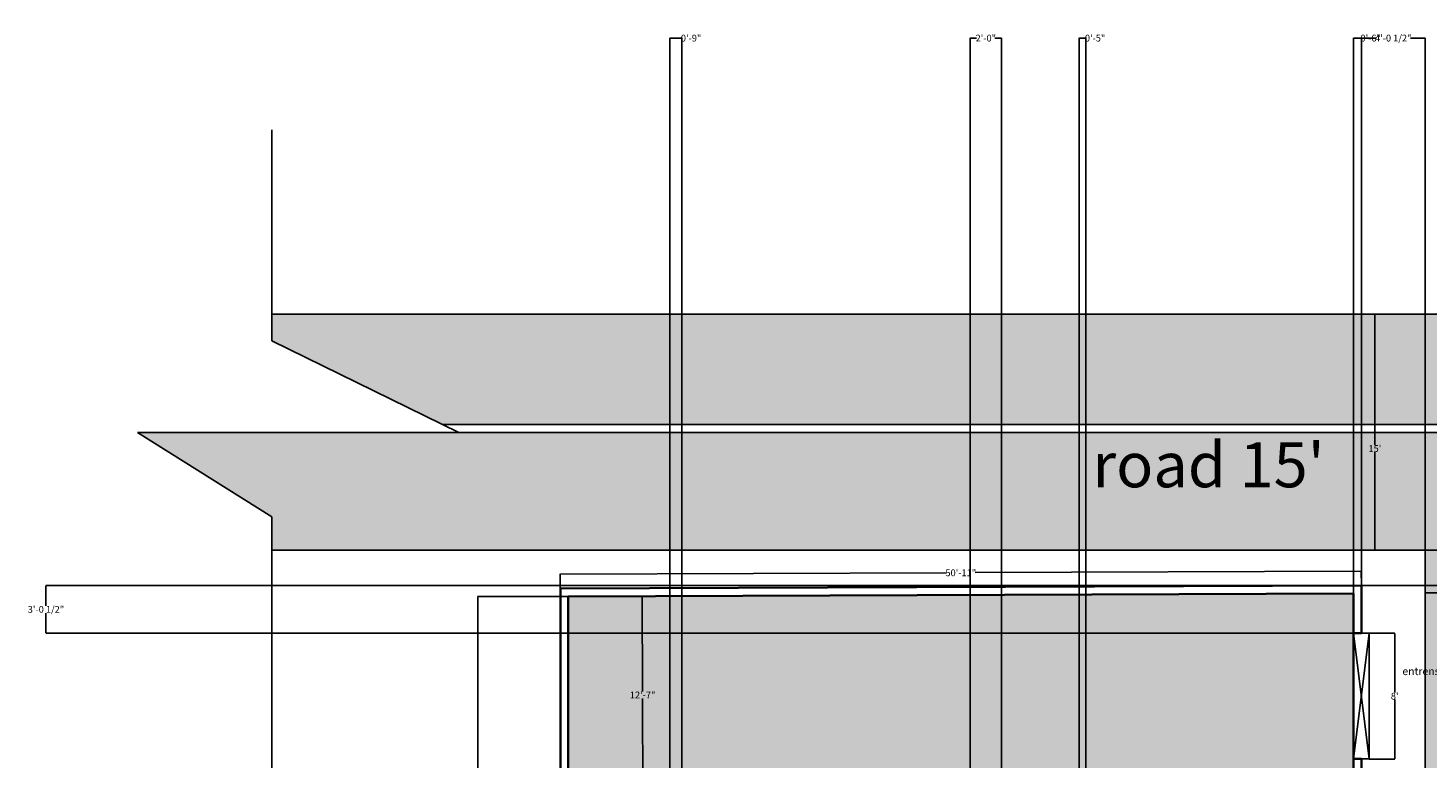
# Model space of a CAD drawing. Units: inches. Extents: x -157 to 1464, y -361 to 1077.
# Tile 8 of 9: x -155 to 913, y 519 to 1077. Entities that reach past the tile are written whole.
import ezdxf

# ---------------------------------------------------------------- set-up
doc = ezdxf.new("R2010")
doc.units = ezdxf.units.IN
doc.header["$MEASUREMENT"] = 0
for name, color, linetype, lineweight in [('A-ANNO-DIMS', 2, 'Continuous', 18), ('C-ANNO-DIMS', 2, 'Continuous', 18), ('C-ANNO-TEXT', 7, 'Continuous', 18), ('C-PROP', 7, 'Continuous', 35), ('C-ROAD', 7, 'Continuous', 25), ('C-ROAD-PATT', 8, 'Continuous', 13), ('C-SITE-GATE', 33, 'Continuous', 25), ('L-GRND-PATT', 8, 'Continuous', 13)]:
    doc.layers.add(name, color=color, linetype=linetype, lineweight=lineweight)
doc.styles.get("Standard").update_dxf_attribs({"font": 'arial.ttf'})
doc.dimstyles.new('Annotative', dxfattribs={"dimscale": 0, "dimtxt": 5.18, "dimasz": 0.18, "dimexe": 0.18, "dimexo": 0.0625, "dimgap": 0.09, "dimtad": 0, "dimtih": 1, "dimtoh": 1, "dimdec": 0, "dimzin": 0, "dimdsep": 46, "dimlunit": 3, "dimtxsty": 'Standard', "dimcen": 0.09, "dimadec": 0, "dimazin": 0, "dimtfac": 1, "dimtdec": 0, "dimtofl": 0, "dimtmove": 0, "dimatfit": 3, "dimfxl": 1, "dimtolj": 1, "dimtzin": 0, "dimarcsym": 0})

# ---------------------------------------------------------------- blocks, each defined once
blk = doc.blocks.new('*D13')
at = {"layer": 'C-ANNO-DIMS', "color": 0, "lineweight": -2, "transparency": 16777216}
for p, q in [((257.3, 643.4), (188.1, 643.4)), ((188.3, 643.2), (188.3, 359.6)), ((188.3, 70.5), (188.3, 354.2)), ((257.3, 70.4), (188.1, 70.4))]:
    blk.add_line(p, q, dxfattribs=at)
at = {"layer": 'C-ANNO-DIMS', "color": 0, "transparency": 16777216}
for points in [[(188.2, 643.2), (188.3, 643.2), (188.3, 643.4)], [(188.2, 70.5), (188.3, 70.5), (188.3, 70.4)]]:
    blk.add_solid(points, dxfattribs=at)
at = {"layer": 'Defpoints', "color": 0, "transparency": 16777216}
for p in [(257.3, 643.4), (188.3, 70.4), (257.3, 70.4)]:
    blk.add_point(p, dxfattribs=at)
at = {"layer": 'C-ANNO-DIMS', "color": 0, "transparency": 16777216, "insert": (188.3, 356.9), "char_height": 5.18, "attachment_point": 5}
blk.add_mtext('\\A1;47\'-9"', dxfattribs=at)
blk = doc.blocks.new('*D17')
at = {"layer": 'C-ANNO-DIMS', "color": 0, "lineweight": -2, "transparency": 16777216}
for p, q in [((868.6, 615.4), (888.2, 615.4)), ((888, 615.2), (888, 570.2)), ((888, 519.6), (888, 564.7)), ((868.6, 519.4), (888.2, 519.4))]:
    blk.add_line(p, q, dxfattribs=at)
at = {"layer": 'C-ANNO-DIMS', "color": 0, "transparency": 16777216}
for points in [[(888, 615.2), (888.1, 615.2), (888, 615.4)], [(888, 519.6), (888.1, 519.6), (888, 519.4)]]:
    blk.add_solid(points, dxfattribs=at)
at = {"layer": 'Defpoints', "color": 0, "transparency": 16777216}
for p in [(868.6, 615.4), (888, 615.4), (868.6, 519.4)]:
    blk.add_point(p, dxfattribs=at)
at = {"layer": 'C-ANNO-DIMS', "color": 0, "transparency": 16777216, "insert": (888, 567.4), "char_height": 5.18, "attachment_point": 5}
blk.add_mtext("\\A1;8'", dxfattribs=at)
blk = doc.blocks.new('*D43')
at = {"layer": 'C-ANNO-DIMS', "color": 0, "lineweight": -2, "transparency": 16777216}
for p, q in [((911.3, 678.8), (911.3, 645.9)), ((1091.3, 678.8), (1091.3, 645.9)), ((911.5, 646.1), (997, 646.1)), ((1091.1, 646.1), (1005.5, 646.1))]:
    blk.add_line(p, q, dxfattribs=at)
at = {"layer": 'C-ANNO-DIMS', "color": 0, "transparency": 16777216}
for points in [[(911.5, 646.1), (911.5, 646), (911.3, 646.1)], [(1091.1, 646.1), (1091.1, 646), (1091.3, 646.1)]]:
    blk.add_solid(points, dxfattribs=at)
at = {"layer": 'Defpoints', "color": 0, "transparency": 16777216}
for p in [(911.3, 678.8), (1091.3, 678.8), (1091.3, 646.1)]:
    blk.add_point(p, dxfattribs=at)
at = {"layer": 'C-ANNO-DIMS', "color": 0, "transparency": 16777216, "insert": (1001.3, 646.1), "char_height": 5.18, "attachment_point": 5}
blk.add_mtext("\\A1;15'", dxfattribs=at)
blk = doc.blocks.new('*D44')
at = {"layer": 'C-ANNO-DIMS', "color": 0, "lineweight": -2, "transparency": 16777216}
for p, q in [((911.2, 858.8), (872.7, 858.8)), ((872.9, 858.7), (872.9, 759.1)), ((872.9, 679), (872.9, 753.6)), ((911.2, 678.8), (872.7, 678.8))]:
    blk.add_line(p, q, dxfattribs=at)
at = {"layer": 'C-ANNO-DIMS', "color": 0, "transparency": 16777216}
for points in [[(872.8, 858.7), (872.9, 858.7), (872.9, 858.8)], [(872.8, 679), (872.9, 679), (872.9, 678.8)]]:
    blk.add_solid(points, dxfattribs=at)
at = {"layer": 'Defpoints', "color": 0, "transparency": 16777216}
for p in [(872.9, 858.8), (911.3, 858.8), (911.3, 678.8)]:
    blk.add_point(p, dxfattribs=at)
at = {"layer": 'C-ANNO-DIMS', "color": 0, "transparency": 16777216, "insert": (872.9, 756.3), "char_height": 5.18, "attachment_point": 5}
blk.add_mtext("\\A1;15'", dxfattribs=at)
blk = doc.blocks.new('*D51')
at = {"layer": 'C-ANNO-DIMS', "color": 0, "lineweight": -2, "transparency": 16777216}
for p, q in [((862.3, 662.7), (567.9, 661.6)), ((862.6, 651.8), (862.5, 662.9)), ((251.3, 649.5), (251.3, 660.6)), ((251.5, 660.4), (545.9, 661.5))]:
    blk.add_line(p, q, dxfattribs=at)
at = {"layer": 'C-ANNO-DIMS', "color": 0, "transparency": 16777216}
for points in [[(862.3, 662.7), (862.3, 662.7), (862.5, 662.7)], [(251.5, 660.4), (251.5, 660.3), (251.3, 660.4)]]:
    blk.add_solid(points, dxfattribs=at)
at = {"layer": 'Defpoints', "color": 0, "transparency": 16777216}
for p in [(251.3, 660.4), (862.6, 651.7), (251.3, 649.4)]:
    blk.add_point(p, dxfattribs=at)
at = {"layer": 'C-ANNO-DIMS', "color": 0, "transparency": 16777216, "insert": (556.9, 661.5), "char_height": 5.18, "attachment_point": 5}
blk.add_mtext('\\A1;50\'-11"', dxfattribs=at)
blk = doc.blocks.new('*D52')
at = {"layer": 'C-ANNO-DIMS', "color": 0, "lineweight": -2, "transparency": 16777216}
for p, q in [((298.5, 643.6), (313.9, 643.6)), ((313.8, 643.5), (314, 571)), ((314.3, 493.1), (314.1, 565.6)), ((299, 492.9), (314.5, 492.9))]:
    blk.add_line(p, q, dxfattribs=at)
at = {"layer": 'C-ANNO-DIMS', "color": 0, "transparency": 16777216}
for points in [[(313.8, 643.5), (313.7, 643.5), (313.8, 643.6)], [(314.4, 493.1), (314.3, 493.1), (314.3, 492.9)]]:
    blk.add_solid(points, dxfattribs=at)
at = {"layer": 'Defpoints', "color": 0, "transparency": 16777216}
for p in [(298.4, 643.6), (313.8, 643.6), (299, 492.9)]:
    blk.add_point(p, dxfattribs=at)
at = {"layer": 'C-ANNO-DIMS', "color": 0, "transparency": 16777216, "insert": (314.1, 568.3), "char_height": 5.18, "attachment_point": 5}
blk.add_mtext('\\A1;12\'-7"', dxfattribs=at)
blk = doc.blocks.new('*D66')
at = {"layer": 'A-ANNO-DIMS', "color": 0, "lineweight": -2, "transparency": 16777216}
for p, q in [((862.5, 651.7), (-141.4, 651.7)), ((-141.2, 651.6), (-141.2, 636.3)), ((-141.2, 615.6), (-141.2, 630.8)), ((868.5, 615.4), (-141.4, 615.4))]:
    blk.add_line(p, q, dxfattribs=at)
at = {"layer": 'A-ANNO-DIMS', "color": 0, "transparency": 16777216}
for points in [[(-141.2, 651.6), (-141.2, 651.6), (-141.2, 651.7)], [(-141.2, 615.6), (-141.2, 615.6), (-141.2, 615.4)]]:
    blk.add_solid(points, dxfattribs=at)
at = {"layer": 'Defpoints', "color": 0, "transparency": 16777216}
for p in [(862.6, 651.7), (-141.2, 615.4), (868.6, 615.4)]:
    blk.add_point(p, dxfattribs=at)
at = {"layer": 'A-ANNO-DIMS', "color": 0, "transparency": 16777216, "insert": (-141.2, 633.6), "char_height": 5.18, "attachment_point": 5}
blk.add_mtext('\\A1;3\'-0 1/2"', dxfattribs=at)
blk = doc.blocks.new('*D67')
at = {"layer": 'A-ANNO-DIMS', "color": 0, "lineweight": -2, "transparency": 16777216}
for p, q in [((862.6, 651.8), (862.6, 1069.7)), ((862.8, 1069.5), (873.8, 1069.5)), ((911.1, 1069.5), (900, 1069.5)), ((911.3, 678.9), (911.3, 1069.7))]:
    blk.add_line(p, q, dxfattribs=at)
at = {"layer": 'A-ANNO-DIMS', "color": 0, "transparency": 16777216}
for points in [[(862.8, 1069.5), (862.8, 1069.5), (862.6, 1069.5)], [(911.1, 1069.5), (911.1, 1069.5), (911.3, 1069.5)]]:
    blk.add_solid(points, dxfattribs=at)
at = {"layer": 'Defpoints', "color": 0, "transparency": 16777216}
for p in [(911.3, 1069.5), (911.3, 678.8), (862.6, 651.7)]:
    blk.add_point(p, dxfattribs=at)
at = {"layer": 'A-ANNO-DIMS', "color": 0, "transparency": 16777216, "insert": (886.9, 1069.5), "char_height": 5.18, "attachment_point": 5}
blk.add_mtext('\\A1;4\'-0 1/2"', dxfattribs=at)
blk = doc.blocks.new('*D68')
at = {"layer": 'A-ANNO-DIMS', "color": 0, "lineweight": -2, "transparency": 16777216}
for p, q in [((911.3, 678.8), (1397.6, 678.8)), ((1397.4, 678.7), (1397.4, 668)), ((1397.4, 651.9), (1397.4, 662.6)), ((862.6, 651.7), (1397.6, 651.7))]:
    blk.add_line(p, q, dxfattribs=at)
at = {"layer": 'A-ANNO-DIMS', "color": 0, "transparency": 16777216}
for points in [[(1397.4, 678.7), (1397.4, 678.7), (1397.4, 678.8)], [(1397.4, 651.9), (1397.4, 651.9), (1397.4, 651.7)]]:
    blk.add_solid(points, dxfattribs=at)
at = {"layer": 'Defpoints', "color": 0, "transparency": 16777216}
for p in [(911.3, 678.8), (1397.4, 678.8), (862.6, 651.7)]:
    blk.add_point(p, dxfattribs=at)
at = {"layer": 'A-ANNO-DIMS', "color": 0, "transparency": 16777216, "insert": (1397.4, 665.3), "char_height": 5.18, "attachment_point": 5}
blk.add_mtext('\\A1;2\'-3"', dxfattribs=at)
blk = doc.blocks.new('*D70')
at = {"layer": 'A-ANNO-DIMS', "color": 0, "lineweight": -2, "transparency": 16777216}
for p, q in [((856.6, 645.8), (856.6, 1069.7)), ((856.8, 1069.5), (862.4, 1069.5)), ((862.6, 651.8), (862.6, 1069.7)), ((862.6, 1069.5), (862.8, 1069.5))]:
    blk.add_line(p, q, dxfattribs=at)
at = {"layer": 'A-ANNO-DIMS', "color": 0, "transparency": 16777216}
for points in [[(856.8, 1069.5), (856.8, 1069.5), (856.6, 1069.5)], [(862.4, 1069.5), (862.4, 1069.5), (862.6, 1069.5)]]:
    blk.add_solid(points, dxfattribs=at)
at = {"layer": 'Defpoints', "color": 0, "transparency": 16777216}
for p in [(862.6, 1069.5), (862.6, 651.7), (856.6, 645.7)]:
    blk.add_point(p, dxfattribs=at)
at = {"layer": 'A-ANNO-DIMS', "color": 0, "transparency": 16777216, "insert": (869.7, 1069.5), "char_height": 5.18, "attachment_point": 5}
blk.add_mtext('\\A1;0\'-6"', dxfattribs=at)
blk = doc.blocks.new('*D80')
at = {"layer": 'A-ANNO-DIMS', "color": 0, "lineweight": -2, "transparency": 16777216}
for p, q in [((335, 492.9), (335, 1069.7)), ((335.1, 1069.5), (343.8, 1069.5)), ((344, 492.9), (344, 1069.7)), ((344, 1069.5), (344.1, 1069.5))]:
    blk.add_line(p, q, dxfattribs=at)
at = {"layer": 'A-ANNO-DIMS', "color": 0, "transparency": 16777216}
for points in [[(335.1, 1069.5), (335.1, 1069.5), (335, 1069.5)], [(343.8, 1069.5), (343.8, 1069.5), (344, 1069.5)]]:
    blk.add_solid(points, dxfattribs=at)
at = {"layer": 'Defpoints', "color": 0, "transparency": 16777216}
for p in [(344, 1069.5), (335, 492.9), (344, 492.9)]:
    blk.add_point(p, dxfattribs=at)
at = {"layer": 'A-ANNO-DIMS', "color": 0, "transparency": 16777216, "insert": (351.1, 1069.5), "char_height": 5.18, "attachment_point": 5}
blk.add_mtext('\\A1;0\'-9"', dxfattribs=at)
blk = doc.blocks.new('*D81')
at = {"layer": 'A-ANNO-DIMS', "color": 0, "lineweight": -2, "transparency": 16777216}
for p, q in [((564, 144.9), (564, 1069.7)), ((564.1, 1069.5), (568.9, 1069.5)), ((587.8, 1069.5), (583, 1069.5)), ((588, 120.9), (588, 1069.7))]:
    blk.add_line(p, q, dxfattribs=at)
at = {"layer": 'A-ANNO-DIMS', "color": 0, "transparency": 16777216}
for points in [[(564.1, 1069.5), (564.1, 1069.5), (564, 1069.5)], [(587.8, 1069.5), (587.8, 1069.5), (588, 1069.5)]]:
    blk.add_solid(points, dxfattribs=at)
at = {"layer": 'Defpoints', "color": 0, "transparency": 16777216}
for p in [(588, 1069.5), (564, 144.9), (588, 120.9)]:
    blk.add_point(p, dxfattribs=at)
at = {"layer": 'A-ANNO-DIMS', "color": 0, "transparency": 16777216, "insert": (576, 1069.5), "char_height": 5.18, "attachment_point": 5}
blk.add_mtext('\\A1;2\'-0"', dxfattribs=at)
blk = doc.blocks.new('*D82')
at = {"layer": 'A-ANNO-DIMS', "color": 0, "lineweight": -2, "transparency": 16777216}
for p, q in [((647.3, 271.1), (647.3, 1069.7)), ((647.4, 1069.5), (652.1, 1069.5)), ((652.3, 276.1), (652.3, 1069.7)), ((652.3, 1069.5), (652.4, 1069.5))]:
    blk.add_line(p, q, dxfattribs=at)
at = {"layer": 'A-ANNO-DIMS', "color": 0, "transparency": 16777216}
for points in [[(647.4, 1069.5), (647.4, 1069.5), (647.3, 1069.5)], [(652.1, 1069.5), (652.1, 1069.5), (652.3, 1069.5)]]:
    blk.add_solid(points, dxfattribs=at)
at = {"layer": 'Defpoints', "color": 0, "transparency": 16777216}
for p in [(652.3, 1069.5), (647.3, 271), (652.3, 276)]:
    blk.add_point(p, dxfattribs=at)
at = {"layer": 'A-ANNO-DIMS', "color": 0, "transparency": 16777216, "insert": (659.4, 1069.5), "char_height": 5.18, "attachment_point": 5}
blk.add_mtext('\\A1;0\'-5"', dxfattribs=at)

msp = doc.modelspace()

# ---------------------------------------------------------------- hatches: boundary and pattern name
at = {"layer": 'C-ROAD-PATT'}
h = msp.add_hatch(color=256, dxfattribs=at)
h.dxf.hatch_style = 1
h.paths.add_polyline_path([(1091.28, 858.84), (31.23, 858.84), (31.23, 838.38), (161.57, 774.56), (996.76, 774.56), (996.76, -105.32), (1027.51, -42.52), (1027.51, -185.11), (1027.51, -287.61), (1091.28, -186.19)])
h.paths.add_polyline_path([(899.55, 208.71), (1098.57, 208.71), (1098.57, 279.4), (899.55, 279.4)], flags=9)
h = msp.add_hatch(color=256, dxfattribs=at)
h.dxf.hatch_style = 1
h.paths.add_polyline_path([(990.76, 768.56), (31.23, 768.56), (-71.27, 768.56), (31.23, 704.11), (31.23, 678.84), (911.28, 678.84), (911.28, -185.11), (957.69, -185.11), (990.76, -117.57)])
h.paths.add_polyline_path([(899.55, 208.71), (1098.57, 208.71), (1098.57, 279.4), (899.55, 279.4)], flags=9)
h.paths.add_polyline_path([(645.57, 707.88), (844.59, 707.88), (844.59, 778.57), (645.57, 778.57)], flags=9)
h.paths.add_polyline_path([(892.1, 580.27), (940.38, 580.27), (940.38, 592.3), (892.1, 592.3)], flags=25)
at = {"layer": 'L-GRND-PATT'}
h = msp.add_hatch(dxfattribs=at)
h.set_pattern_fill('GRAVEL', color=256, scale=26)
h.set_pattern_definition([(228.01279, (18.72, 26), (-208, -234), [3.49794, -346.2963]), (184.96974, (16.38, 23.4), (312, 26), [6.00257, -594.25404]), (132.51045, (10.4, 22.88), (260, -286), [4.2325, -419.01685]), (267.27369, (0.26, 16.38), (26, 520), [5.4662, -541.1525]), (292.83365, (0, 10.92), (-130, 312), [5.36003, -530.6437]), (357.27369, (2.08, 5.98), (-520, 26), [5.4662, -541.1525]), (37.69424, (7.54, 5.72), (-338, -260), [7.22875, -715.64606]), (72.25533, (13.26, 10.14), (182, 572), [6.8247, -675.64436]), (121.42957, (15.34, 16.64), (-208, 338), [5.4847, -542.9859]), (175.23636, (12.48, 21.32), (286, -26), [6.26163, -306.81983]), (222.39744, (6.24, 21.84), (-312, -286), [8.09765, -801.66775]), (138.81407, (26, 16.12), (-182, 156), [2.76383, -273.61997]), (171.46923, (23.92, 17.94), (338, -52), [5.25816, -520.5593]), (225, (18.72, 18.72), (-3e-15, -26), [3.67695, -33.0926]), (203.1986, (16.9, 21.84), (130, 52), [1.9801, -196.03]), (291.8014, (15.08, 21.06), (-26, 78), [2.8003, -137.214]), (30.96376, (16.12, 18.46), (78, 52), [4.54815, -147.0566]), (161.56505, (20.02, 20.8), (52, -26), [3.28877, -78.93045]), (16.38954, (0, 21.06), (260, 78), [4.6072, -456.11397]), (70.34618, (4.42, 22.36), (-104, -286), [3.8652, -382.6526]), (293.1986, (20.02, 26), (-52, 130), [3.9602, -194.0499]), (343.61046, (21.58, 22.36), (-260, 78), [4.6072, -456.11397]), (339.44395, (0, 4.94), (-130, 52), [4.4429, -217.7012]), (294.77514, (4.16, 3.38), (-130, 286), [3.72263, -368.5407]), (66.8014, (20.28, 0), (52, 130), [3.9602, -194.0499]), (17.35402, (21.84, 3.64), (-338, -104), [4.3584, -431.481]), (69.44395, (7.54, 0), (-52, -130), [2.22144, -219.92266]), (101.30993, (18.72, 0), (-26, 104), [1.32574, -131.24877]), (165.96376, (18.46, 1.3), (78, -26), [5.36003, -101.8407]), (186.009, (13.26, 2.6), (260, 26), [4.9673, -491.762]), (303.6901, (16.12, 16.12), (-26, 52), [3.7498, -89.99456]), (353.15723, (18.2, 13), (442, -52), [6.54664, -648.11663]), (60.9454, (24.7, 12.22), (-104, -182), [2.67686, -265.00953]), (90, (26, 14.56), (-26, 26), [1.56, -24.44]), (120.25644, (12.74, 3.38), (104, -182), [3.61202, -357.5915]), (48.01279, (10.92, 6.5), (208, 234), [6.99587, -342.79835]), (0, (15.6, 11.7), (26, 26), [6.76, -19.24]), (325.30485, (22.36, 11.7), (260, -182), [4.11096, -406.98513]), (254.0546, (25.74, 9.36), (-26, -104), [3.78565, -185.4972]), (207.64598, (24.7, 5.72), (-494, -260), [6.1637, -610.20633]), (175.42608, (19.24, 2.86), (-338, 26), [6.52077, -645.5559])])
h.paths.add_polyline_path([(856.57, 645.71), (257.33, 643.42), (257.33, 70.37), (856.57, 72.66)])
h.paths.add_polyline_path([(668.97, 111.86), (596.97, 111.86), (298.97, 111.86), (298.97, 420.86), (298.97, 492.86), (427.97, 492.86), (668.97, 492.86)], flags=16)
h.paths.add_polyline_path([(842.44, 305.24), (842.44, 199.78), (692.18, 199.78), (692.18, 305.24)], flags=16)
h.paths.add_polyline_path([(596.97, 369.86), (596.97, 158.9), (587.97, 158.9), (587.97, 120.86), (485.97, 120.86), (485.97, 203.86), (468.97, 203.86), (468.97, 198.86), (480.97, 198.86), (480.97, 120.86), (465.97, 120.86), (465.97, 111.86), (447.97, 111.86), (447.97, 120.86), (432.97, 120.86), (432.97, 198.86), (438.97, 198.86), (438.97, 203.86), (432.97, 203.86), (432.97, 226.86), (427.97, 226.86), (427.97, 120.86), (307.97, 120.86), (307.97, 146.36), (298.97, 146.36), (298.97, 194.36), (307.97, 194.36), (307.97, 267.86), (427.97, 267.86), (427.97, 262.86), (432.97, 262.86), (432.97, 277.86), (427.97, 277.86), (427.97, 272.86), (307.97, 272.86), (307.97, 276.53), (298.97, 276.53), (298.97, 324.53), (307.97, 324.53), (307.97, 411.86), (427.97, 411.86), (427.97, 313.86), (432.97, 313.86), (432.97, 411.86), (463.95, 411.86), (463.95, 420.86), (334.97, 420.86), (334.97, 456.86), (427.97, 456.86), (427.97, 420.86), (546.97, 420.86), (582.97, 420.86), (596.97, 420.86), (596.97, 405.86)], flags=0)
h.paths.add_polyline_path([(596.97, 369.86), (587.97, 369.86), (587.97, 324), (596.97, 324), (596.97, 276), (587.97, 276), (587.97, 369.86), (587.97, 405.86), (587.97, 411.86), (582.97, 411.86), (546.97, 411.86), (546.97, 420.86), (564.97, 416.36), (582.97, 420.86), (582.97, 411.86), (587.97, 411.86), (587.97, 405.86), (596.97, 405.86), (592.47, 387.86)], flags=0)
h.paths.add_polyline_path([(468.97, 203.86), (468.97, 198.86), (438.97, 198.86), (438.97, 203.86)], flags=0)
h.paths.add_polyline_path([(267.35, 260.99), (288.37, 260.99), (288.37, 271.66), (267.35, 271.66)], flags=24)
h.paths.add_polyline_path([(435.51, 88.48), (460.55, 88.48), (460.55, 99.15), (435.51, 99.15)], flags=24)
h.paths.add_polyline_path([(315.69, 188.99), (336.72, 188.99), (336.72, 199.66), (315.69, 199.66)], flags=8)
h.paths.add_polyline_path([(361.73, 141.9), (373.75, 141.9), (373.75, 152.57), (361.73, 152.57)], flags=8)
h.paths.add_polyline_path([(430.38, 154.49), (447.38, 154.49), (447.38, 165.16), (430.38, 165.16)], flags=8)
h.paths.add_polyline_path([(451.09, 165.32), (468.09, 165.32), (468.09, 175.99), (451.09, 175.99)], flags=8)
h.paths.add_polyline_path([(361.73, 305.06), (373.75, 305.06), (373.75, 315.74), (361.73, 315.74)], flags=8)
h.paths.add_polyline_path([(316.13, 336.94), (337.15, 336.94), (337.15, 347.62), (316.13, 347.62)], flags=8)
h.paths.add_polyline_path([(484.07, 423.56), (492.07, 423.56), (492.07, 434.24), (484.07, 434.24)], flags=8)
h.paths.add_polyline_path([(560.99, 428.52), (568.98, 428.52), (568.98, 439.19), (560.99, 439.19)], flags=8)
h.paths.add_polyline_path([(528.49, 131.95), (545.49, 131.95), (545.49, 142.62), (528.49, 142.62)], flags=8)
h.paths.add_polyline_path([(564.53, 188.99), (585.55, 188.99), (585.55, 199.66), (564.53, 199.66)], flags=8)

# ---------------------------------------------------------------- linework, layer by layer
at = {"layer": 'C-PROP'}
for p, q in [((856.57, 615.42), (862.57, 615.42)), ((856.57, 519.42), (862.57, 519.42))]:
    msp.add_line(p, q, dxfattribs=at)
msp.add_lwpolyline([(862.57, 615.42), (862.57, 651.74), (251.33, 649.4), (251.33, 64.34), (862.57, 66.68), (862.57, 519.42)], dxfattribs=at)
msp.add_lwpolyline([(257.33, 70.37), (856.57, 72.66), (856.57, 645.71), (257.33, 643.42)], close=True, dxfattribs=at)
at = {"layer": 'C-ROAD'}
for p, q in [((31.23, 838.38), (31.23, 999.54)), ((31.23, 858.84), (1091.28, 858.84)), ((173.83, 768.56), (31.23, 838.38)), ((161.57, 774.56), (996.76, 774.56)), ((31.23, 768.56), (-71.27, 768.56)), ((-71.27, 768.56), (31.23, 704.11)), ((31.23, 768.56), (990.76, 768.56)), ((31.23, 468.62), (31.23, 704.11)), ((31.23, 678.84), (911.28, 678.84)), ((911.28, 678.84), (911.28, -185.11))]:
    msp.add_line(p, q, dxfattribs=at)
at = {"layer": 'C-SITE-GATE'}
for p, q in [((856.57, 615.42), (868.57, 615.42)), ((856.57, 615.42), (868.57, 519.42)), ((868.57, 615.42), (856.57, 519.42)), ((856.57, 519.42), (856.57, 615.42)), ((868.57, 519.42), (868.57, 615.42)), ((856.57, 519.42), (868.57, 519.42))]:
    msp.add_line(p, q, dxfattribs=at)

# ---------------------------------------------------------------- texts
at = {"layer": 'C-ANNO-TEXT', "attachment_point": 1}
for s, width, gutter_width, heights, insert, char_height in [("{\\fArial|b1|i0|c0|p34;road 15'}", 513.204, 171.53, [77.1], (657.31, 761.05), 34.3055), ('entrens gate', 87.358, 29.2, [13.12], (893.86, 589.3), 5.8395)]:
    msp.add_mtext_dynamic_manual_height_columns(s, width=width, gutter_width=gutter_width, heights=heights, dxfattribs=dict(at, insert=insert, char_height=char_height))

# ---------------------------------------------------------------- dimensions: what is measured, and where the dimension line sits
at = {"layer": 'A-ANNO-DIMS'}
for base, p1, p2, picture, middle in [((343.97, 1069.48), (334.97, 492.86), (343.97, 492.86), '*D80', (351.12, 1069.48)), ((587.97, 1069.48), (563.97, 144.86), (587.97, 120.86), '*D81', (575.97, 1069.48)), ((652.25, 1069.48), (647.25, 271), (652.25, 276), '*D82', (659.4, 1069.48)), ((862.57, 1069.48), (856.57, 645.71), (862.57, 651.74), '*D70', (869.72, 1069.48)), ((911.28, 1069.48), (862.57, 651.74), (911.28, 678.84), '*D67', (886.93, 1069.48))]:
    dim = msp.add_linear_dim(base=base, p1=p1, p2=p2, dimstyle='Annotative', override={"dimscale": 1, "dimdec": 1, "dimzin": 1, "dimlunit": 4, "dimfrac": 2}, dxfattribs=at)
    dim.commit()
    dim.dimension.update_dxf_attribs({"geometry": picture, "text_midpoint": middle})
for base, p2, picture, middle in [((1397.39, 678.84), (911.28, 678.84), '*D68', (1397.39, 665.29)), ((-141.21, 615.42), (868.57, 615.42), '*D66', (-141.21, 633.58))]:
    dim = msp.add_linear_dim(base=base, p1=(862.57, 651.74), p2=p2, angle=90, dimstyle='Annotative', override={"dimscale": 1, "dimdec": 1, "dimzin": 1, "dimlunit": 4, "dimfrac": 2}, dxfattribs=at)
    dim.commit()
    dim.dimension.update_dxf_attribs({"geometry": picture, "text_midpoint": middle})
at = {"layer": 'C-ANNO-DIMS'}
dim = msp.add_linear_dim(base=(872.88, 858.84), p1=(911.28, 678.84), p2=(911.28, 858.84), angle=90, dimstyle='Annotative', override={"dimclrd": 0, "dimclre": 0, "dimclrt": 0}, dxfattribs=at)
dim.commit()
dim.dimension.update_dxf_attribs({"geometry": '*D44', "text_midpoint": (872.88, 756.34), "dimtype": 160})
dim = msp.add_linear_dim(base=(1091.28, 646.07), p1=(911.28, 678.84), p2=(1091.28, 678.84), dimstyle='Annotative', override={"dimclrd": 0, "dimclre": 0, "dimclrt": 0}, dxfattribs=at)
dim.commit()
dim.dimension.update_dxf_attribs({"geometry": '*D43', "text_midpoint": (1001.28, 646.07)})
for p1, p2, distance, picture, middle in [((862.57, 651.74), (251.33, 649.4), -10.97, '*D51', (556.91, 661.54)), ((298.97, 492.86), (298.39, 643.58), -15.38, '*D52', (314.05, 568.28))]:
    dim = msp.add_aligned_dim(p1=p1, p2=p2, distance=distance, dimstyle='Annotative', override={"dimclrd": 0, "dimclre": 0, "dimclrt": 0}, dxfattribs=at)
    dim.commit()
    dim.dimension.update_dxf_attribs({"geometry": picture, "text_midpoint": middle})
for base, p1, p2, picture, middle in [((188.26, 70.37), (257.33, 643.42), (257.33, 70.37), '*D13', (188.26, 356.89)), ((888.03, 615.42), (868.57, 519.42), (868.57, 615.42), '*D17', (888.03, 567.42))]:
    dim = msp.add_linear_dim(base=base, p1=p1, p2=p2, angle=90, dimstyle='Annotative', override={"dimclrd": 0, "dimclre": 0, "dimclrt": 0}, dxfattribs=at)
    dim.commit()
    dim.dimension.update_dxf_attribs({"geometry": picture, "text_midpoint": middle})

doc.saveas('drawing.dxf')
